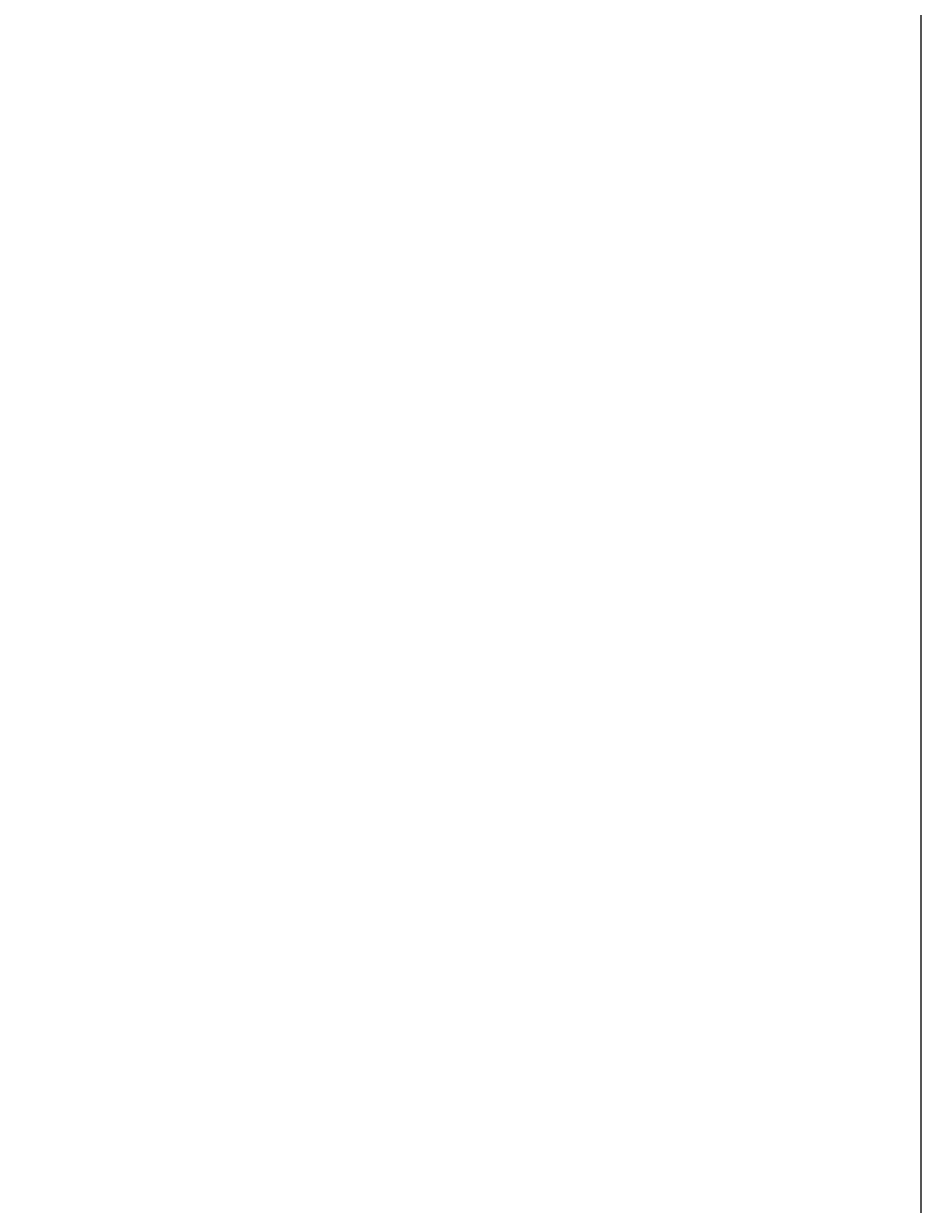
# Model space of a CAD drawing. Units: inches. Extents: x 1568 to 2529, y 2149 to 2897.
# Tile 8 of 16: x 1974 to 2010, y 2364 to 2410. Entities that reach past the tile are written whole.
import ezdxf

# ---------------------------------------------------------------- set-up
doc = ezdxf.new("R2010")
doc.units = ezdxf.units.IN
doc.layers.add('A-ANNO-DIMS', color=2, linetype='Continuous', lineweight=18)
doc.styles.get("Standard").update_dxf_attribs({"font": 'arial.ttf'})
doc.dimstyles.get("Standard").update_dxf_attribs({"dimtxt": 0.18, "dimasz": 0.18, "dimexe": 0.18, "dimexo": 0.0625, "dimgap": 0.09, "dimtad": 0, "dimtih": 1, "dimtoh": 1, "dimdec": 4, "dimzin": 0, "dimdsep": 46, "dimtxsty": 'Standard', "dimcen": 0.09, "dimadec": 0, "dimazin": 0, "dimtfac": 1, "dimtdec": 4, "dimtofl": 0, "dimtmove": 0, "dimatfit": 3, "dimfxl": 1, "dimtolj": 1, "dimtzin": 0, "dimarcsym": 0})

# ---------------------------------------------------------------- blocks, each defined once
blk = doc.blocks.new('*D28')
at = {"layer": 'A-ANNO-DIMS', "color": 0, "lineweight": -2, "transparency": 16777216}
for p, q in [((1973.643, 2801.532), (2009.61, 2801.532)), ((2009.43, 2801.352), (2009.43, 2501.714)), ((2009.43, 2201.712), (2009.43, 2501.35)), ((1973.613, 2201.532), (2009.61, 2201.532))]:
    blk.add_line(p, q, dxfattribs=at)
at = {"layer": 'A-ANNO-DIMS', "color": 0, "transparency": 16777216}
for points in [[(2009.4, 2801.352), (2009.46, 2801.352), (2009.43, 2801.532)], [(2009.4, 2201.712), (2009.46, 2201.712), (2009.43, 2201.532)]]:
    blk.add_solid(points, dxfattribs=at)
at = {"layer": 'Defpoints', "color": 0, "transparency": 16777216}
for p in [(1973.58, 2801.532), (2009.43, 2801.532), (1973.551, 2201.532)]:
    blk.add_point(p, dxfattribs=at)
at = {"layer": 'A-ANNO-DIMS', "color": 0, "transparency": 16777216, "insert": (2009.43, 2501.532), "char_height": 0.18, "attachment_point": 5}
blk.add_mtext('\\A1;600', dxfattribs=at)

msp = doc.modelspace()

# ---------------------------------------------------------------- dimensions: what is measured, and where the dimension line sits
at = {"layer": 'A-ANNO-DIMS'}
dim = msp.add_linear_dim(base=(2009.4302, 2801.532), p1=(1973.5509, 2201.532), p2=(1973.5802, 2801.532), angle=90, dimstyle='Standard', override={"dimdec": 0, "dimlfac": 1, "dimrnd": 0, "dimzin": 0, "dimdsep": 46, "dimlunit": 2}, dxfattribs=at)
dim.commit()
dim.dimension.update_dxf_attribs({"geometry": '*D28', "text_midpoint": (2009.4302, 2501.532)})

doc.saveas('drawing.dxf')
